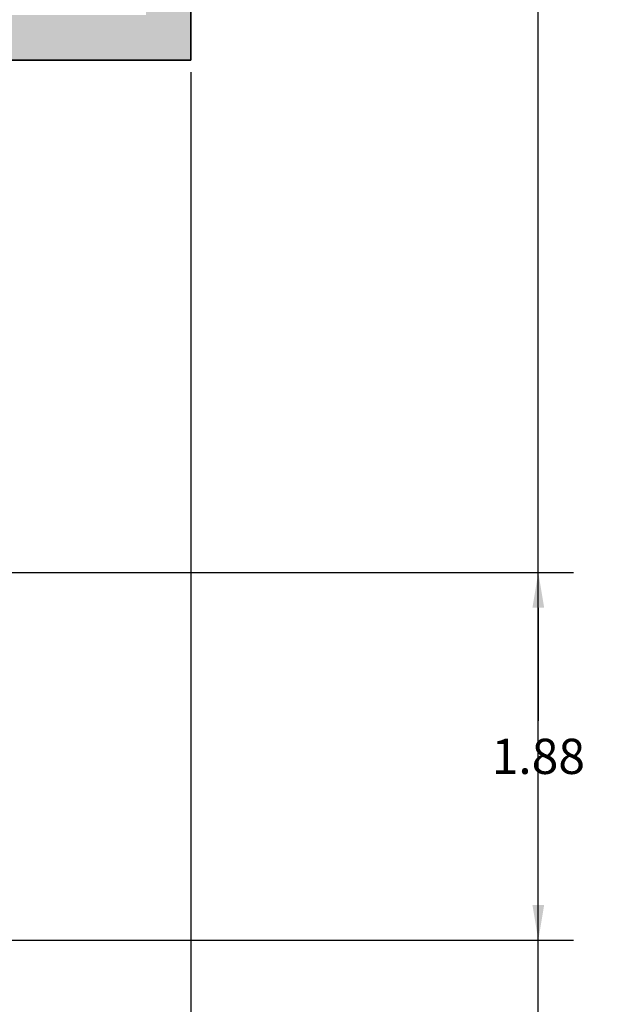
# Model space of a CAD drawing. Units: metres. Extents: x 4298.5 to 4325.2, y 2075 to 2095.8.
# Tile 31 of 35: x 4321.9 to 4324.9, y 2079.7 to 2084.8. Entities that reach past the tile are written whole.
import ezdxf

# ---------------------------------------------------------------- set-up
doc = ezdxf.new("R2010")
doc.units = ezdxf.units.M
for name, color, linetype, lineweight in [('A-ANNO-DIMS', 2, 'Continuous', 18), ('A-WALL', 7, 'Continuous', 35), ('A-WALL-PATT', 252, 'Continuous', 13)]:
    doc.layers.add(name, color=color, linetype=linetype, lineweight=lineweight)
doc.styles.get("Standard").update_dxf_attribs({"font": 'arial.ttf'})
doc.dimstyles.get("Standard").update_dxf_attribs({"dimtxt": 0.18, "dimasz": 0.18, "dimexe": 0.18, "dimexo": 0.0625, "dimgap": 0.09, "dimtad": 0, "dimtih": 1, "dimtoh": 1, "dimdec": 4, "dimzin": 0, "dimdsep": 46, "dimtxsty": 'Standard', "dimcen": 0.09, "dimadec": 0, "dimazin": 0, "dimtfac": 1, "dimtdec": 4, "dimtofl": 0, "dimtmove": 0, "dimatfit": 3, "dimfxl": 1, "dimtolj": 1, "dimtzin": 0, "dimarcsym": 0})

# ---------------------------------------------------------------- blocks, each defined once
blk = doc.blocks.new('*D47')
at = {"layer": 'A-ANNO-DIMS', "color": 0, "lineweight": -2, "transparency": 16777216}
for p, q in [((4300.4306, 2084.4956), (4300.4306, 2074.9896)), ((4322.8106, 2084.4956), (4322.8106, 2074.9896)), ((4300.6106, 2075.1696), (4311.2252, 2075.1696)), ((4322.6306, 2075.1696), (4312.016, 2075.1696))]:
    blk.add_line(p, q, dxfattribs=at)
at = {"layer": 'A-ANNO-DIMS', "color": 0, "transparency": 16777216}
for points in [[(4300.6106, 2075.1996), (4300.6106, 2075.1396), (4300.4306, 2075.1696)], [(4322.6306, 2075.1996), (4322.6306, 2075.1396), (4322.8106, 2075.1696)]]:
    blk.add_solid(points, dxfattribs=at)
at = {"layer": 'Defpoints', "color": 0, "transparency": 16777216}
for p in [(4300.4306, 2084.5581), (4322.8106, 2084.5581), (4322.8106, 2075.1696)]:
    blk.add_point(p, dxfattribs=at)
at = {"layer": 'A-ANNO-DIMS', "color": 0, "transparency": 16777216, "insert": (4311.6206, 2075.1696), "char_height": 0.18, "attachment_point": 5}
blk.add_mtext('\\A1;22.38', dxfattribs=at)
blk = doc.blocks.new('*D48')
at = {"layer": 'A-ANNO-DIMS', "color": 0, "lineweight": -2, "transparency": 16777216}
for p, q in [((4310.1831, 2094.4781), (4324.7671, 2094.4781)), ((4324.5871, 2094.2981), (4324.5871, 2085.585)), ((4324.5871, 2076.5081), (4324.5871, 2085.2212)), ((4316.8731, 2076.3281), (4324.7671, 2076.3281))]:
    blk.add_line(p, q, dxfattribs=at)
at = {"layer": 'A-ANNO-DIMS', "color": 0, "transparency": 16777216}
for points in [[(4324.5571, 2094.2981), (4324.6171, 2094.2981), (4324.5871, 2094.4781)], [(4324.5571, 2076.5081), (4324.6171, 2076.5081), (4324.5871, 2076.3281)]]:
    blk.add_solid(points, dxfattribs=at)
at = {"layer": 'Defpoints', "color": 0, "transparency": 16777216}
for p in [(4310.1206, 2094.4781), (4316.8106, 2076.3281), (4324.5871, 2076.3281)]:
    blk.add_point(p, dxfattribs=at)
at = {"layer": 'A-ANNO-DIMS', "color": 0, "transparency": 16777216, "insert": (4324.5871, 2085.4031), "char_height": 0.18, "attachment_point": 5}
blk.add_mtext('\\A1;18.15', dxfattribs=at)
blk = doc.blocks.new('*D55')
at = {"layer": 'A-ANNO-DIMS', "color": 0, "lineweight": -2, "transparency": 16777216}
for p, q in [((4320.3167, 2084.4996), (4320.3167, 2074.9896)), ((4322.8106, 2084.4956), (4322.8106, 2074.9896)), ((4320.4967, 2075.1696), (4321.1688, 2075.1696)), ((4322.6306, 2075.1696), (4321.9585, 2075.1696))]:
    blk.add_line(p, q, dxfattribs=at)
at = {"layer": 'A-ANNO-DIMS', "color": 0, "transparency": 16777216}
for points in [[(4320.4967, 2075.1996), (4320.4967, 2075.1396), (4320.3167, 2075.1696)], [(4322.6306, 2075.1996), (4322.6306, 2075.1396), (4322.8106, 2075.1696)]]:
    blk.add_solid(points, dxfattribs=at)
at = {"layer": 'Defpoints', "color": 0, "transparency": 16777216}
for p in [(4320.3167, 2084.5621), (4322.8106, 2084.5581), (4322.8106, 2075.1696)]:
    blk.add_point(p, dxfattribs=at)
at = {"layer": 'A-ANNO-DIMS', "color": 0, "transparency": 16777216, "insert": (4321.5636, 2075.1696), "char_height": 0.18, "attachment_point": 5}
blk.add_mtext('\\A1;2.494', dxfattribs=at)
blk = doc.blocks.new('*D60')
at = {"layer": 'A-ANNO-DIMS', "color": 0, "lineweight": -2, "transparency": 16777216}
for p, q in [((4305.9531, 2081.9381), (4324.7671, 2081.9381)), ((4324.5871, 2081.7581), (4324.5871, 2081.18)), ((4324.5871, 2080.2381), (4324.5871, 2080.8162)), ((4305.9531, 2080.0581), (4324.7671, 2080.0581))]:
    blk.add_line(p, q, dxfattribs=at)
at = {"layer": 'A-ANNO-DIMS', "color": 0, "transparency": 16777216}
for points in [[(4324.5571, 2081.7581), (4324.6171, 2081.7581), (4324.5871, 2081.9381)], [(4324.5571, 2080.2381), (4324.6171, 2080.2381), (4324.5871, 2080.0581)]]:
    blk.add_solid(points, dxfattribs=at)
at = {"layer": 'Defpoints', "color": 0, "transparency": 16777216}
for p in [(4305.8906, 2081.9381), (4324.5871, 2081.9381), (4305.8906, 2080.0581)]:
    blk.add_point(p, dxfattribs=at)
at = {"layer": 'A-ANNO-DIMS', "color": 0, "transparency": 16777216, "insert": (4324.5871, 2080.9981), "char_height": 0.18, "attachment_point": 5}
blk.add_mtext('\\A1;1.88', dxfattribs=at)

msp = doc.modelspace()

# ---------------------------------------------------------------- hatches: boundary and pattern name
at = {"layer": 'A-WALL-PATT'}
h = msp.add_hatch(color=256, dxfattribs=at)
h.dxf.hatch_style = 1
h.paths.add_polyline_path([(4308.7606, 2094.4781), (4308.1606, 2094.4781), (4307.4606, 2094.4781), (4307.4606, 2094.2481), (4308.2706, 2094.2481), (4308.2706, 2094.1281), (4308.3906, 2094.1281), (4308.3906, 2094.2481), (4308.7606, 2094.2481)])
h.paths.add_polyline_path([(4310.1206, 2094.4781), (4309.5206, 2094.4781), (4309.5206, 2094.2481), (4309.8906, 2094.2481), (4309.8906, 2092.2481), (4308.3906, 2092.2481), (4308.3906, 2093.4281), (4308.2706, 2093.4281), (4308.2706, 2092.0181), (4309.8906, 2092.0181), (4309.8906, 2087.0181), (4309.7706, 2087.0181), (4309.7706, 2086.7881), (4309.8906, 2086.7881), (4311.9406, 2086.7881), (4311.9406, 2087.0181), (4310.1206, 2087.0181), (4310.1206, 2089.0181), (4310.2406, 2089.0181), (4310.2406, 2089.1381), (4310.1206, 2089.1381), (4310.1206, 2092.0181), (4310.3078, 2092.0181), (4310.3078, 2092.2481), (4310.1206, 2092.2481)])
h.paths.add_polyline_path([(4311.7406, 2092.2481), (4311.0678, 2092.2481), (4311.0678, 2092.0181), (4311.7406, 2092.0181)], flags=17)
h.paths.add_polyline_path([(4313.1733, 2092.2481), (4312.5006, 2092.2481), (4312.5006, 2092.0181), (4313.1733, 2092.0181)])
h.paths.add_polyline_path([(4314.5378, 2092.2481), (4314.1206, 2092.2481), (4313.9333, 2092.2481), (4313.9333, 2092.0181), (4314.1206, 2092.0181), (4314.1206, 2087.0181), (4314.0006, 2087.0181), (4314.0006, 2086.7881), (4314.1206, 2086.7881), (4315.5718, 2086.7881), (4315.5718, 2087.0181), (4314.3506, 2087.0181), (4314.3506, 2092.0181), (4314.5378, 2092.0181)])
h.paths.add_polyline_path([(4315.9706, 2092.2481), (4315.2978, 2092.2481), (4315.2978, 2092.0181), (4315.9706, 2092.0181)])
h.paths.add_polyline_path([(4317.4033, 2092.2481), (4316.7306, 2092.2481), (4316.7306, 2092.0181), (4317.4033, 2092.0181)])
h.paths.add_polyline_path([(4318.9506, 2092.2481), (4318.3506, 2092.2481), (4318.1633, 2092.2481), (4318.1633, 2092.0181), (4318.3506, 2092.0181), (4318.3506, 2091.8981), (4318.5806, 2091.8981), (4318.5806, 2092.0181), (4318.9506, 2092.0181)])
h.paths.add_polyline_path([(4321.0106, 2092.2481), (4319.7106, 2092.2481), (4319.7106, 2092.0181), (4320.0806, 2092.0181), (4320.0806, 2090.0181), (4318.5806, 2090.0181), (4318.5806, 2091.1981), (4318.3506, 2091.1981), (4318.3506, 2090.0181), (4318.3506, 2087.0181), (4318.2306, 2087.0181), (4318.2306, 2086.7881), (4318.3506, 2086.7881), (4318.3506, 2086.3081), (4318.5806, 2086.3081), (4318.5806, 2089.7881), (4321.7806, 2089.7881), (4321.7806, 2090.0181), (4320.2006, 2090.0181), (4320.2006, 2092.0181), (4321.0106, 2092.0181)])
h.paths.add_polyline_path([(4322.8106, 2092.2481), (4321.7706, 2092.2481), (4321.7706, 2092.0181), (4322.5806, 2092.0181), (4322.5806, 2091.2831), (4322.8106, 2091.2831)])
h.paths.add_polyline_path([(4322.8106, 2090.5231), (4322.5806, 2090.5231), (4322.5806, 2089.7881), (4322.5806, 2089.5254), (4322.8106, 2089.5254), (4322.8106, 2090.0181)])
h.paths.add_polyline_path([(4322.8106, 2088.7654), (4322.5806, 2088.7654), (4322.5806, 2087.6681), (4322.8106, 2087.6681)])
h.paths.add_polyline_path([(4322.8106, 2086.9081), (4322.5806, 2086.9081), (4322.5806, 2085.8107), (4322.8106, 2085.8107)])
h.paths.add_polyline_path([(4322.8106, 2085.0507), (4322.5806, 2085.0507), (4322.5806, 2084.7881), (4318.5806, 2084.7881), (4318.5806, 2085.0581), (4318.5806, 2085.4081), (4318.3506, 2085.4081), (4318.3506, 2084.5581), (4318.3506, 2080.8581), (4318.4706, 2080.8581), (4318.4706, 2082.3281), (4319.2606, 2082.3281), (4319.2606, 2082.5581), (4318.5806, 2082.5581), (4318.5806, 2084.5581), (4320.0806, 2084.5581), (4320.0806, 2083.9381), (4320.3106, 2083.9381), (4320.3106, 2084.5581), (4322.8106, 2084.5581)])
h.paths.add_polyline_path([(4320.3106, 2083.1781), (4320.0806, 2083.1781), (4320.0806, 2082.5581), (4319.9606, 2082.5581), (4319.9606, 2082.3281), (4320.0806, 2082.3281), (4320.0806, 2081.5731), (4320.3106, 2081.5731)], flags=17)
h.paths.add_polyline_path([(4320.3106, 2080.8131), (4320.0806, 2080.8131), (4320.0806, 2080.0581), (4318.4286, 2080.0581), (4318.4286, 2079.8281), (4320.3106, 2079.8281)])
h.paths.add_polyline_path([(4317.3506, 2085.2881), (4316.5718, 2085.2881), (4316.5718, 2085.0581), (4317.3506, 2085.0581)])
h.paths.add_polyline_path([(4315.5718, 2085.2881), (4314.8434, 2085.2881), (4314.8434, 2085.0581), (4315.5718, 2085.0581)])
h.paths.add_polyline_path([(4313.8434, 2085.2881), (4312.9406, 2085.2881), (4312.9406, 2085.0581), (4313.8434, 2085.0581)])
h.paths.add_polyline_path([(4311.9406, 2085.2881), (4311.4406, 2085.2881), (4311.4406, 2085.0581), (4311.9406, 2085.0581)])
h.paths.add_polyline_path([(4317.3306, 2087.0181), (4316.5718, 2087.0181), (4316.5718, 2086.7881), (4317.3306, 2086.7881)])
h.paths.add_polyline_path([(4313.1006, 2089.1381), (4311.1406, 2089.1381), (4311.1406, 2089.0181), (4312.9806, 2089.0181), (4312.9806, 2087.0181), (4312.9406, 2087.0181), (4312.9406, 2086.7881), (4313.1006, 2086.7881), (4313.1006, 2087.0181)])
h.paths.add_polyline_path([(4307.5515, 2087.0181), (4305.8906, 2087.0181), (4305.8906, 2092.2481), (4305.8906, 2094.2481), (4306.7006, 2094.2481), (4306.7006, 2094.4781), (4305.6606, 2094.4781), (4305.6606, 2092.2481), (4305.2906, 2092.2481), (4305.2906, 2092.0181), (4305.6606, 2092.0181), (4305.6606, 2090.0181), (4304.1606, 2090.0181), (4304.1606, 2091.1981), (4304.0406, 2091.1981), (4304.0406, 2089.9081), (4301.5606, 2089.9081), (4301.5606, 2089.7881), (4304.0406, 2089.7881), (4305.6606, 2089.7881), (4305.6606, 2086.6381), (4305.8906, 2086.6381), (4305.8906, 2086.7881), (4307.5515, 2086.7881)])
h.paths.add_polyline_path([(4307.5515, 2085.2881), (4305.8906, 2085.2881), (4305.8906, 2085.4381), (4305.6606, 2085.4381), (4305.6606, 2084.7881), (4305.2906, 2084.7881), (4305.2906, 2084.5581), (4305.6606, 2084.5581), (4305.6606, 2084.02), (4305.8906, 2084.02), (4305.8906, 2084.5581), (4305.8906, 2085.0581), (4307.5515, 2085.0581)])
h.paths.add_polyline_path([(4310.2406, 2085.2881), (4308.5515, 2085.2881), (4308.5515, 2085.0581), (4310.2406, 2085.0581)])
h.paths.add_polyline_path([(4317.4286, 2080.0581), (4316.5718, 2080.0581), (4316.5718, 2079.8281), (4317.4286, 2079.8281)])
h.paths.add_polyline_path([(4315.5718, 2080.0581), (4314.8434, 2080.0581), (4314.8434, 2079.8281), (4315.5718, 2079.8281)])
h.paths.add_polyline_path([(4313.8434, 2080.0581), (4312.9406, 2080.0581), (4312.9406, 2079.8281), (4313.8434, 2079.8281)])
h.paths.add_polyline_path([(4311.9406, 2080.0581), (4311.4406, 2080.0581), (4311.4406, 2079.8281), (4311.9406, 2079.8281)])
h.paths.add_polyline_path([(4310.2406, 2080.0581), (4310.1206, 2080.0581), (4310.1206, 2084.0381), (4309.8906, 2084.0381), (4309.8906, 2080.0581), (4309.1606, 2080.0581), (4309.1606, 2079.8281), (4310.2406, 2079.8281)])
h.paths.add_polyline_path([(4308.1606, 2080.0581), (4307.5106, 2080.0581), (4307.5106, 2080.1781), (4307.3906, 2080.1781), (4307.3906, 2080.0581), (4305.8906, 2080.0581), (4305.8906, 2080.567), (4305.6606, 2080.567), (4305.6606, 2079.8281), (4308.1606, 2079.8281)])
h.paths.add_polyline_path([(4307.5106, 2081.9381), (4309.0906, 2081.9381), (4309.0906, 2082.0581), (4305.8906, 2082.0581), (4305.8906, 2083.26), (4305.6606, 2083.26), (4305.6606, 2081.327), (4305.8906, 2081.327), (4305.8906, 2081.9381), (4307.3906, 2081.9381), (4307.3906, 2080.8781), (4307.5106, 2080.8781)])
h.paths.add_polyline_path([(4304.5306, 2084.7881), (4302.7306, 2084.7881), (4302.7306, 2084.5581), (4304.5306, 2084.5581)])
h.paths.add_polyline_path([(4301.9706, 2084.7881), (4300.6606, 2084.7881), (4300.6606, 2085.0249), (4300.4306, 2085.0249), (4300.4306, 2084.5581), (4301.9706, 2084.5581)])
h.paths.add_polyline_path([(4300.6606, 2086.8843), (4300.4306, 2086.8843), (4300.4306, 2085.7849), (4300.6606, 2085.7849)])
h.paths.add_polyline_path([(4300.6606, 2089.1618), (4300.4306, 2089.1618), (4300.4306, 2087.6443), (4300.6606, 2087.6443)])
h.paths.add_polyline_path([(4300.6606, 2091.0212), (4300.4306, 2091.0212), (4300.4306, 2089.9218), (4300.6606, 2089.9218)])
h.paths.add_polyline_path([(4300.6606, 2092.0181), (4301.9706, 2092.0181), (4301.9706, 2092.2481), (4300.4306, 2092.2481), (4300.4306, 2091.7812), (4300.6606, 2091.7812)])
h.paths.add_polyline_path([(4304.5306, 2092.2481), (4302.7306, 2092.2481), (4302.7306, 2092.0181), (4304.0406, 2092.0181), (4304.0406, 2091.8981), (4304.1606, 2091.8981), (4304.1606, 2092.0181), (4304.5306, 2092.0181)], flags=17)

# ---------------------------------------------------------------- linework, layer by layer
at = {"layer": 'A-WALL'}
for p, q in [((4322.8106, 2090.0181), (4322.8106, 2084.5581)), ((4322.8106, 2084.5581), (4320.3106, 2084.5581))]:
    msp.add_line(p, q, dxfattribs=at)

# ---------------------------------------------------------------- dimensions: what is measured, and where the dimension line sits
at = {"layer": 'A-ANNO-DIMS'}
for base, p1, p2, picture, middle in [((4324.5871, 2076.3281), (4310.1206, 2094.4781), (4316.8106, 2076.3281), '*D48', (4324.5871, 2085.4031)), ((4324.5871, 2081.9381), (4305.8906, 2080.0581), (4305.8906, 2081.9381), '*D60', (4324.5871, 2080.9981))]:
    dim = msp.add_linear_dim(base=base, p1=p1, p2=p2, angle=90, dimstyle='Standard', override={"dimdec": 2, "dimlfac": 1, "dimrnd": 0, "dimzin": 0, "dimdsep": 46, "dimlunit": 2}, dxfattribs=at)
    dim.commit()
    dim.dimension.update_dxf_attribs({"geometry": picture, "text_midpoint": middle})
for p1, override, picture, middle in [((4300.4306, 2084.5581), {"dimdec": 2, "dimlfac": 1, "dimrnd": 0, "dimzin": 0, "dimdsep": 46, "dimlunit": 2}, '*D47', (4311.6206, 2075.1696)), ((4320.3167, 2084.5621), {"dimdec": 3, "dimlfac": 1, "dimrnd": 0, "dimzin": 0, "dimdsep": 46, "dimlunit": 2}, '*D55', (4321.5636, 2075.1696))]:
    dim = msp.add_linear_dim(base=(4322.8106, 2075.1696), p1=p1, p2=(4322.8106, 2084.5581), dimstyle='Standard', override=override, dxfattribs=at)
    dim.commit()
    dim.dimension.update_dxf_attribs({"geometry": picture, "text_midpoint": middle})

doc.saveas('drawing.dxf')
